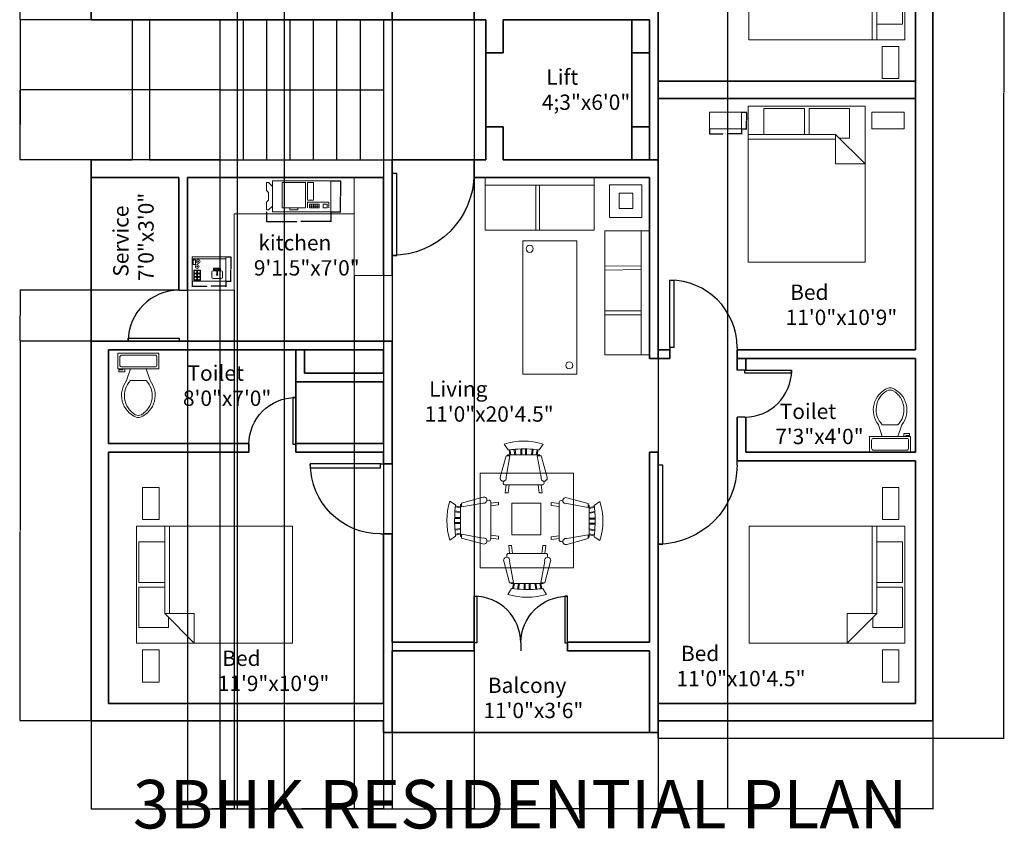
# Model space of a CAD drawing. Units: inches. Extents: x 108 to 613, y 1573 to 2319.
# Tile 1 of 11: x 108 to 613, y 1573 to 1989. Entities that reach past the tile are written whole.
import ezdxf

# ---------------------------------------------------------------- set-up
doc = ezdxf.new("R2010")
doc.units = ezdxf.units.IN
for name, color, linetype, lineweight in [('A-ANNO-DIMS', 2, 'Continuous', 18), ('A-AREA-IDEN', 3, 'Continuous', 18), ('A-EQPM', 2, 'Continuous', 18), ('A-FLOR-CASE', 6, 'Continuous', 18), ('A-FLOR-FIXT', 2, 'Continuous', 18), ('door', 4, 'Continuous', 25), ('furniture', 2, 'Continuous', 18), ('staircase', 7, 'Continuous', 25), ('text', 7, 'Continuous', 25), ('wall', 6, 'Continuous', 35)]:
    doc.layers.add(name, color=color, linetype=linetype, lineweight=lineweight)
doc.styles.get("Standard").update_dxf_attribs({"font": 'arial.ttf'})
doc.dimstyles.get("Standard").update_dxf_attribs({"dimtxt": 0.18, "dimasz": 0.18, "dimexe": 0.18, "dimexo": 0.0625, "dimgap": 0.09, "dimtad": 0, "dimtih": 1, "dimtoh": 1, "dimdec": 4, "dimzin": 0, "dimdsep": 46, "dimtxsty": 'Standard', "dimcen": 0.09, "dimadec": 0, "dimazin": 0, "dimtfac": 1, "dimtdec": 4, "dimtofl": 0, "dimtmove": 0, "dimatfit": 3, "dimfxl": 1, "dimtolj": 1, "dimtzin": 0, "dimarcsym": 0})

# ---------------------------------------------------------------- blocks, each defined once
blk = doc.blocks.new('*U2')
for p, q in [((0, 0), (0, -5)), ((30, 0), (30, -5))]:
    blk.add_line(p, q)
blk.add_lwpolyline([(0, 0), (0, 30), (1.75, 30), (1.75, 0)], close=True)
blk.add_arc((0, 0), 30, 0, 90)
blk = doc.blocks.new('Bed - Queen')
for p, q in [((0, -80.00003), (0, 0)), ((0, 0), (59.99999, 0)), ((59.99999, 0), (59.99999, -80.00003)), ((7.99999, -1.2), (28.79998, -1.2)), ((7.99999, -14.4), (7.99999, -1.2)), ((28.79998, -1.2), (28.79998, -14.4)), ((31.19999, -1.2), (51.99999, -1.2)), ((31.19999, -14.4), (31.19999, -1.2)), ((51.99999, -1.2), (51.99999, -16.4)), ((0, -14.4), (44.8, -14.4)), ((59.99999, -29.6), (44.8, -14.4)), ((44.8, -14.4), (44.8, -29.6)), ((44.8, -16.8), (0, -16.8)), ((51.99999, -16.4), (46.79936, -16.4)), ((44.8, -29.6), (59.99999, -29.6)), ((59.99999, -80.00003), (0, -80.00003))]:
    blk.add_line(p, q)
blk = doc.blocks.new('Copy Machine')
for p, q in [((0, 0), (0, -16)), ((30, 0), (0, 0)), ((30, -16), (30, 0)), ((-3, -1), (-3, -5)), ((-2, -1), (-3, -1)), ((-3, -5), (-2, -6)), ((0, -3), (-2, -1)), ((5, -1), (5, -14)), ((17, -1), (5, -1)), ((17, -14), (17, -1)), ((18, -1), (18, -10)), ((21, -1), (18, -1)), ((21, -10), (21, -1)), ((-3, -11), (-2, -10)), ((-2, -10), (-2, -6)), ((18, -10), (21, -10)), ((-3, -15), (-3, -11)), ((-2, -15), (-3, -15)), ((0, -13), (-2, -15)), ((5, -14), (17, -14)), ((9, -14), (9, -15)), ((9, -15), (13, -15)), ((13, -15), (13, -14)), ((18, -14), (18, -11)), ((18, -11), (29, -11)), ((24, -12), (19, -12)), ((19, -12), (19, -14)), ((24, -13), (19, -13)), ((19, -14), (24, -14)), ((20, -12), (20, -14)), ((21, -14), (21, -12)), ((22, -12), (22, -14)), ((23, -14), (23, -12)), ((24, -14), (24, -12)), ((28, -12), (26, -12)), ((26, -12), (26, -14)), ((26, -14), (28, -14)), ((28, -14), (28, -12)), ((29, -11), (29, -14)), ((0, -16), (30, -16))]:
    blk.add_line(p, q)
blk = doc.blocks.new('Wet Bar')
for p, q in [((0, 0), (36, 0)), ((0, -26), (0, 0)), ((36, 0), (36, -26)), ((0, -2), (36, -2)), ((3.5, -3), (1, -3)), ((1, -3), (1, -8)), ((1, -8), (3.5, -8)), ((3.5, -8), (3.5, -3)), ((2, -14.25), (9, -14.25)), ((2, -24.75), (2, -14.25)), ((2, -17.75), (9, -17.75)), ((5.5, -14.25), (5.5, -24.75)), ((9, -14.25), (9, -24.75)), ((26.2, -17.55), (26.2, -14.1284)), ((27.1001, -17.55), (27.1001, -14.1284)), ((36, -26), (0, -26)), ((9, -21.25), (2, -21.25)), ((9, -24.75), (2, -24.75))]:
    blk.add_line(p, q)
for points in [[(20.95, -21.75), (20.95, -16.05)], [(22.15, -14.85), (26.2, -14.85)], [(26.2, -14.25), (22.95, -14.25), (22.95, -12.2), (26.75, -12.2)], [(26.7487, -12.2), (30.3501, -12.2), (30.3501, -14.25), (27.1001, -14.25)], [(27.1001, -14.85), (31.15, -14.85)], [(32.3501, -16.05), (32.3501, -21.75)], [(31.15, -22.95), (22.15, -22.95)]]:
    blk.add_lwpolyline(points)
for centre, radius in [((5.5, -10.25), 2), ((6.5, -5), 2), ((5.5, -10.25), 0.5), ((6.5, -5), 0.5), ((3.75, -16), 1.5), ((3.75, -19.5), 1.5), ((7.25, -16), 1.5), ((7.25, -19.5), 1.5), ((24.25, -13.25), 0.5), ((26.65, -13.35), 0.9), ((26.65, -19.05), 0.6), ((29, -13.25), 0.5), ((3.75, -23), 1.5), ((7.25, -23), 1.5)]:
    blk.add_circle(centre, radius)
for centre, radius, start, end in [((22.2251, -16.125), 1.2772, 93.36646, 176.6335), ((26.65, -17.55), 0.45, 180, 0), ((31.075, -16.125), 1.2772, 3.366461, 86.63354), ((22.2251, -21.675), 1.2772, 183.3665, 266.6335), ((31.075, -21.675), 1.2772, 273.3665, 356.6335)]:
    blk.add_arc(centre, radius, start, end)
blk = doc.blocks.new('Toilet - top')
for p, q in [((9.5, -6), (9.5, -2)), ((-10, -8.5), (-8, -8.5)), ((-10, -9.5), (-10, -8.5)), ((-7, -9.5), (-10, -9.5)), ((-8, -8.5), (-8, -8)), ((-7, -8), (-7, -9.5)), ((-4, -8), (-6, -14)), ((4, -8), (6, -14)), ((4, -14), (-4, -14))]:
    blk.add_line(p, q)
blk.add_lwpolyline([(10.5, -8), (10.5, 0), (-10.5, 0), (-10.5, -8)], close=True)
for points in [[(-9.5, -2), (-9.5, -6)], [(8.5, -1), (-8.5, -1)], [(-8.5, -7), (8.5, -7)]]:
    blk.add_lwpolyline(points)
for centre, radius, start, end in [((-8.62, -1.88), 0.884, 81.8699, 188.1301), ((8.62, -1.88), 0.884, 351.8699, 98.1301), ((-8.62, -6.12), 0.884, 171.8699, 278.1301), ((8.62, -6.12), 0.884, 261.8699, 8.1301), ((3.52, -21.58), 12.17, 141.4691, 247.9714), ((4.2, -21.82), 11.33, 136.3677, 238.9468), ((-3.52, -21.58), 12.17, 292.0284, 38.5307), ((-4.2, -21.82), 11.33, 301.053, 43.6321), ((0, -27.88), 4, 245.7318, 294.2682), ((0, -29), 4, 254.8605, 285.1395)]:
    blk.add_arc(centre, radius, start, end)
blk = doc.blocks.new('Chair - Rocking')
for p, q in [((-8, -4.5), (-10, -1.5)), ((-7.5, -4.5), (-7, -7)), ((-6.5, -7), (-7.02225, -4.43)), ((-4.5, -7), (-4.96674, -4.19951)), ((-4, -7), (-4.40532, -4.16272)), ((-1.5, -4.05012), (-1.5, -7)), ((-1, -7), (-1, -4.05012)), ((1, -7), (1, -4.04655)), ((1.5, -4.05012), (1.5, -7)), ((4, -7), (4.40187, -4.18694)), ((4.5, -7), (4.96761, -4.19437)), ((6.5, -7), (7, -4.4057)), ((7.5, -4.5), (7, -7)), ((8, -4.5), (10, -1.5)), ((-9, -7.5), (-12, -18.49999)), ((-7, -7.5), (-9, -7.5)), ((-9, -18.49999), (-7, -7.5)), ((-8.23428, -6.99939), (-8.3093, -7.47958)), ((-8.23041, -7), (8.23915, -7)), ((7, -7.5), (9, -7.5)), ((9, -18.49999), (7, -7.5)), ((8.31071, -7.48854), (8.23449, -7.00073)), ((9, -7.5), (12, -18.49999)), ((-10.36644, -20.64523), (-10.5, -21.49999)), ((-9, -22.49999), (-9.5, -26.49999)), ((0, -22.49999), (-9.5, -22.49999)), ((-8, -26.49999), (-7.5, -22.49999)), ((0, -22.49999), (9.5, -22.49999)), ((8, -26.49999), (7.5, -22.49999)), ((9, -22.49999), (9.5, -26.49999)), ((10.5, -21.49999), (10.3575, -20.58798)), ((-9.5, -26.49999), (-8, -26.49999)), ((9.5, -26.49999), (8, -26.49999))]:
    blk.add_line(p, q)
for centre, radius, start, end in [((0, -34.08333), 34.08333, 72.93847, 107.0615), ((0, -68.25004), 64.25, 93.92211, 97.15267), ((0, -68.25004), 64.25, 82.84733, 93.92211), ((-10.5, -18.99999), 1.58114, 161.5651, 18.43495), ((10.5, -18.99999), 1.58114, 161.5651, 18.43495), ((-9.5, -21.49999), 1, 180, 270), ((9.5, -21.49999), 1, 270, 0)]:
    blk.add_arc(centre, radius, start, end)
blk = doc.blocks.new('NIGHTSTAND')
blk.add_lwpolyline([(0, 8.48), (16.5, 8.48), (16.5, 0), (0, 0)], close=True)
blk = doc.blocks.new('COFFEE-TABLE')
blk.add_lwpolyline([(0, 68.46), (27.63, 68.46), (27.63, 0), (0, 0)], close=True)
for centre, radius in [((23.79, 63.93), 1.79), ((3.47, 4.05), 1.83)]:
    blk.add_circle(centre, radius)
blk = doc.blocks.new('SOFA-3-SEAT')
for p, q in [((18.7, 63.66), (18.7, 0)), ((0.03, 43.08), (18.7, 43.08)), ((0.03, 41.08), (18.7, 41.08)), ((0, 18.17), (18.7, 17.89)), ((0.03, 20.17), (18.7, 19.89))]:
    blk.add_line(p, q)
blk.add_lwpolyline([(0.03, 63.66), (22.97, 63.66), (22.97, 0), (0.03, 0)], close=True)
blk = doc.blocks.new('SOFA-2-SEAT')
for p, q in [((25.99, 27.08), (25.99, 4.03)), ((27.99, 27.08), (27.99, 4.03)), ((55.98, 4.03), (0, 4.03))]:
    blk.add_line(p, q)
blk.add_lwpolyline([(0, 27.08), (55.98, 27.08), (55.98, 0), (0, 0)], close=True)
blk = doc.blocks.new('END-TABLE')
for points in [[(0, 16.91), (16.47, 16.91), (16.47, 0), (0, 0)], [(4.92, 12.21), (11.85, 12.21), (11.85, 4.34), (4.92, 4.34)]]:
    blk.add_lwpolyline(points, close=True)
blk = doc.blocks.new('DINING-TABLE')
for points in [[(0, 48.71), (48.06, 48.71), (48.06, 0), (0, 0)], [(16.26, 33.17), (31.3, 33.17), (31.3, 16.93), (16.26, 16.93)]]:
    blk.add_lwpolyline(points, close=True)
blk = doc.blocks.new('*D17')
at = {"layer": 'A-ANNO-DIMS', "color": 0, "lineweight": -2, "transparency": 16777216}
for p, q in [((462.07, 1932.51), (462.07, 1929.91)), ((478.57, 1932.51), (478.57, 1929.91)), ((462.25, 1930.09), (468.94, 1930.09)), ((478.39, 1930.09), (471.7, 1930.09))]:
    blk.add_line(p, q, dxfattribs=at)
at = {"layer": 'A-ANNO-DIMS', "color": 0, "transparency": 16777216}
for points in [[(462.25, 1930.12), (462.25, 1930.06), (462.07, 1930.09)], [(478.39, 1930.12), (478.39, 1930.06), (478.57, 1930.09)]]:
    blk.add_solid(points, dxfattribs=at)
at = {"layer": 'Defpoints', "color": 0, "transparency": 16777216}
for p in [(462.07, 1932.57), (478.57, 1932.57), (478.57, 1930.09)]:
    blk.add_point(p, dxfattribs=at)
at = {"layer": 'A-ANNO-DIMS', "color": 0, "transparency": 16777216, "insert": (470.32, 1930.09), "char_height": 0.18, "attachment_point": 5}
blk.add_mtext('\\A1;NIGHTSTAND 17 TYP.', dxfattribs=at)
blk = doc.blocks.new('*D18')
at = {"layer": 'A-ANNO-DIMS', "color": 0, "lineweight": -2, "transparency": 16777216}
for p, q in [((478.63, 1941.05), (481.23, 1941.05)), ((481.05, 1940.87), (481.05, 1936.99)), ((481.05, 1932.75), (481.05, 1936.63)), ((478.63, 1932.57), (481.23, 1932.57))]:
    blk.add_line(p, q, dxfattribs=at)
at = {"layer": 'A-ANNO-DIMS', "color": 0, "transparency": 16777216}
for points in [[(481.02, 1940.87), (481.08, 1940.87), (481.05, 1941.05)], [(481.02, 1932.75), (481.08, 1932.75), (481.05, 1932.57)]]:
    blk.add_solid(points, dxfattribs=at)
at = {"layer": 'Defpoints', "color": 0, "transparency": 16777216}
for p in [(478.57, 1941.05), (481.05, 1941.05), (478.57, 1932.57)]:
    blk.add_point(p, dxfattribs=at)
at = {"layer": 'A-ANNO-DIMS', "color": 0, "transparency": 16777216, "insert": (481.05, 1936.81), "char_height": 0.18, "attachment_point": 5}
blk.add_mtext('\\A1;8 TYP.', dxfattribs=at)
blk = doc.blocks.new('*D25')
at = {"layer": 'A-ANNO-DIMS', "color": 0, "lineweight": -2, "transparency": 16777216}
for p, q in [((234.84, 1889.9), (234.84, 1884.83)), ((267.84, 1889.9), (267.84, 1884.83)), ((235.02, 1885.01), (250.3, 1885.01)), ((267.66, 1885.01), (252.38, 1885.01))]:
    blk.add_line(p, q, dxfattribs=at)
at = {"layer": 'A-ANNO-DIMS', "color": 0, "transparency": 16777216}
for points in [[(235.02, 1885.04), (235.02, 1884.98), (234.84, 1885.01)], [(267.66, 1885.04), (267.66, 1884.98), (267.84, 1885.01)]]:
    blk.add_solid(points, dxfattribs=at)
at = {"layer": 'Defpoints', "color": 0, "transparency": 16777216}
for p in [(234.84, 1889.96), (267.84, 1889.96), (267.84, 1885.01)]:
    blk.add_point(p, dxfattribs=at)
at = {"layer": 'A-ANNO-DIMS', "color": 0, "transparency": 16777216, "insert": (251.34, 1885.01), "char_height": 0.18, "attachment_point": 5}
blk.add_mtext('\\A1;COPIER 33 TYP.', dxfattribs=at)
blk = doc.blocks.new('*D26')
at = {"layer": 'A-ANNO-DIMS', "color": 0, "lineweight": -2, "transparency": 16777216}
for p, q in [((267.9, 1905.96), (272.97, 1905.96)), ((272.79, 1905.78), (272.79, 1898.14)), ((272.79, 1890.14), (272.79, 1897.78)), ((267.9, 1889.96), (272.97, 1889.96))]:
    blk.add_line(p, q, dxfattribs=at)
at = {"layer": 'A-ANNO-DIMS', "color": 0, "transparency": 16777216}
for points in [[(272.76, 1905.78), (272.82, 1905.78), (272.79, 1905.96)], [(272.76, 1890.14), (272.82, 1890.14), (272.79, 1889.96)]]:
    blk.add_solid(points, dxfattribs=at)
at = {"layer": 'Defpoints', "color": 0, "transparency": 16777216}
for p in [(267.84, 1905.96), (272.79, 1905.96), (267.84, 1889.96)]:
    blk.add_point(p, dxfattribs=at)
at = {"layer": 'A-ANNO-DIMS', "color": 0, "transparency": 16777216, "insert": (272.79, 1897.96), "char_height": 0.18, "attachment_point": 5}
blk.add_mtext('\\A1;16 TYP.', dxfattribs=at)
blk = doc.blocks.new('*D27')
at = {"layer": 'A-ANNO-DIMS', "color": 0, "lineweight": -2, "transparency": 16777216}
for p, q in [((196.59, 1854.26), (196.59, 1851.54)), ((196.77, 1851.72), (204.13, 1851.72)), ((213.76, 1851.72), (206.4, 1851.72)), ((213.94, 1854.26), (213.94, 1851.54))]:
    blk.add_line(p, q, dxfattribs=at)
at = {"layer": 'A-ANNO-DIMS', "color": 0, "transparency": 16777216}
for points in [[(196.77, 1851.75), (196.77, 1851.69), (196.59, 1851.72)], [(213.76, 1851.75), (213.76, 1851.69), (213.94, 1851.72)]]:
    blk.add_solid(points, dxfattribs=at)
at = {"layer": 'Defpoints', "color": 0, "transparency": 16777216}
for p in [(196.59, 1854.32), (213.94, 1854.32), (213.94, 1851.72)]:
    blk.add_point(p, dxfattribs=at)
at = {"layer": 'A-ANNO-DIMS', "color": 0, "transparency": 16777216, "insert": (205.27, 1851.72), "char_height": 0.18, "attachment_point": 5}
blk.add_mtext('\\A1;WET BAR 17 TYP.', dxfattribs=at)
blk = doc.blocks.new('*D28')
at = {"layer": 'A-ANNO-DIMS', "color": 0, "lineweight": -2, "transparency": 16777216}
for p, q in [((214, 1866.85), (216.72, 1866.85)), ((216.54, 1866.67), (216.54, 1860.77)), ((216.54, 1854.5), (216.54, 1860.4)), ((214, 1854.32), (216.72, 1854.32))]:
    blk.add_line(p, q, dxfattribs=at)
at = {"layer": 'A-ANNO-DIMS', "color": 0, "transparency": 16777216}
for points in [[(216.51, 1866.67), (216.57, 1866.67), (216.54, 1866.85)], [(216.51, 1854.5), (216.57, 1854.5), (216.54, 1854.32)]]:
    blk.add_solid(points, dxfattribs=at)
at = {"layer": 'Defpoints', "color": 0, "transparency": 16777216}
for p in [(213.94, 1866.85), (216.54, 1866.85), (213.94, 1854.32)]:
    blk.add_point(p, dxfattribs=at)
at = {"layer": 'A-ANNO-DIMS', "color": 0, "transparency": 16777216, "insert": (216.54, 1860.59), "char_height": 0.18, "attachment_point": 5}
blk.add_mtext('\\A1;13 TYP.', dxfattribs=at)
blk = doc.blocks.new('*D39')
at = {"layer": 'A-ANNO-DIMS', "color": 0, "lineweight": -2, "transparency": 16777216}
for p, q in [((144.78, 1628.55), (144.78, 1583.23)), ((576.78, 1628.55), (576.78, 1583.23)), ((144.96, 1583.41), (360.48, 1583.41)), ((576.6, 1583.41), (361.07, 1583.41))]:
    blk.add_line(p, q, dxfattribs=at)
at = {"layer": 'A-ANNO-DIMS', "color": 0, "transparency": 16777216}
for points in [[(144.96, 1583.44), (144.96, 1583.38), (144.78, 1583.41)], [(576.6, 1583.44), (576.6, 1583.38), (576.78, 1583.41)]]:
    blk.add_solid(points, dxfattribs=at)
at = {"layer": 'Defpoints', "color": 0, "transparency": 16777216}
for p in [(144.78, 1628.61), (576.78, 1628.61), (576.78, 1583.41)]:
    blk.add_point(p, dxfattribs=at)
at = {"layer": 'A-ANNO-DIMS', "color": 0, "transparency": 16777216, "insert": (360.78, 1583.41), "char_height": 0.18, "attachment_point": 5}
blk.add_mtext('\\A1;432', dxfattribs=at)
blk = doc.blocks.new('*D40')
at = {"layer": 'A-ANNO-DIMS', "color": 0, "lineweight": -2, "transparency": 16777216}
for p, q in [((435.84, 2282.61), (613.31, 2282.61)), ((613.13, 2282.43), (613.13, 1951.37)), ((613.13, 1619.94), (613.13, 1951.01)), ((435.84, 1619.76), (613.31, 1619.76))]:
    blk.add_line(p, q, dxfattribs=at)
at = {"layer": 'A-ANNO-DIMS', "color": 0, "transparency": 16777216}
for points in [[(613.1, 2282.43), (613.16, 2282.43), (613.13, 2282.61)], [(613.1, 1619.94), (613.16, 1619.94), (613.13, 1619.76)]]:
    blk.add_solid(points, dxfattribs=at)
at = {"layer": 'Defpoints', "color": 0, "transparency": 16777216}
for p in [(435.78, 2282.61), (613.13, 2282.61), (435.78, 1619.76)]:
    blk.add_point(p, dxfattribs=at)
at = {"layer": 'A-ANNO-DIMS', "color": 0, "transparency": 16777216, "insert": (613.13, 1951.19), "char_height": 0.18, "attachment_point": 5}
blk.add_mtext('\\A1;662.8', dxfattribs=at)
blk = doc.blocks.new('*D43')
at = {"layer": 'A-ANNO-DIMS', "color": 0, "lineweight": -2, "transparency": 16777216}
for p, q in [((144.71, 1823.61), (108.25, 1823.61)), ((108.43, 1823.43), (108.43, 1726.29)), ((108.43, 1628.79), (108.43, 1725.93)), ((144.71, 1628.61), (108.25, 1628.61))]:
    blk.add_line(p, q, dxfattribs=at)
at = {"layer": 'A-ANNO-DIMS', "color": 0, "transparency": 16777216}
for points in [[(108.4, 1823.43), (108.46, 1823.43), (108.43, 1823.61)], [(108.4, 1628.79), (108.46, 1628.79), (108.43, 1628.61)]]:
    blk.add_solid(points, dxfattribs=at)
at = {"layer": 'Defpoints', "color": 0, "transparency": 16777216}
for p in [(108.43, 1823.61), (144.78, 1823.61), (144.78, 1628.61)]:
    blk.add_point(p, dxfattribs=at)
at = {"layer": 'A-ANNO-DIMS', "color": 0, "transparency": 16777216, "insert": (108.43, 1726.11), "char_height": 0.18, "attachment_point": 5}
blk.add_mtext('\\A1;195', dxfattribs=at)
blk = doc.blocks.new('*D44')
at = {"layer": 'A-ANNO-DIMS', "color": 0, "lineweight": -2, "transparency": 16777216}
for p, q in [((144.71, 1988.61), (108.25, 1988.61)), ((108.43, 1988.43), (108.43, 1952.79)), ((108.43, 1916.79), (108.43, 1952.43)), ((144.71, 1916.61), (108.25, 1916.61))]:
    blk.add_line(p, q, dxfattribs=at)
at = {"layer": 'A-ANNO-DIMS', "color": 0, "transparency": 16777216}
for points in [[(108.4, 1988.43), (108.46, 1988.43), (108.43, 1988.61)], [(108.4, 1916.79), (108.46, 1916.79), (108.43, 1916.61)]]:
    blk.add_solid(points, dxfattribs=at)
at = {"layer": 'Defpoints', "color": 0, "transparency": 16777216}
for p in [(108.43, 1988.61), (144.78, 1988.61), (144.78, 1916.61)]:
    blk.add_point(p, dxfattribs=at)
at = {"layer": 'A-ANNO-DIMS', "color": 0, "transparency": 16777216, "insert": (108.43, 1952.61), "char_height": 0.18, "attachment_point": 5}
blk.add_mtext('\\A1;72', dxfattribs=at)
blk = doc.blocks.new('*D45')
at = {"layer": 'A-ANNO-DIMS', "color": 0, "lineweight": -2, "transparency": 16777216}
for p, q in [((144.71, 2276.61), (108.25, 2276.61)), ((108.43, 2276.43), (108.43, 2132.79)), ((108.43, 1988.79), (108.43, 2132.43)), ((144.71, 1988.61), (108.25, 1988.61))]:
    blk.add_line(p, q, dxfattribs=at)
at = {"layer": 'A-ANNO-DIMS', "color": 0, "transparency": 16777216}
for points in [[(108.4, 2276.43), (108.46, 2276.43), (108.43, 2276.61)], [(108.4, 1988.79), (108.46, 1988.79), (108.43, 1988.61)]]:
    blk.add_solid(points, dxfattribs=at)
at = {"layer": 'Defpoints', "color": 0, "transparency": 16777216}
for p in [(108.43, 2276.61), (144.78, 2276.61), (144.78, 1988.61)]:
    blk.add_point(p, dxfattribs=at)
at = {"layer": 'A-ANNO-DIMS', "color": 0, "transparency": 16777216, "insert": (108.43, 2132.61), "char_height": 0.18, "attachment_point": 5}
blk.add_mtext('\\A1;288', dxfattribs=at)
blk = doc.blocks.new('*D48')
at = {"layer": 'A-ANNO-DIMS', "color": 0, "lineweight": -2, "transparency": 16777216}
for p, q in [((299.28, 1988.55), (299.28, 1583.23)), ((341.28, 1988.55), (341.28, 1583.23)), ((299.46, 1583.41), (320.05, 1583.41)), ((341.1, 1583.41), (320.5, 1583.41))]:
    blk.add_line(p, q, dxfattribs=at)
at = {"layer": 'A-ANNO-DIMS', "color": 0, "transparency": 16777216}
for points in [[(299.46, 1583.44), (299.46, 1583.38), (299.28, 1583.41)], [(341.1, 1583.44), (341.1, 1583.38), (341.28, 1583.41)]]:
    blk.add_solid(points, dxfattribs=at)
at = {"layer": 'Defpoints', "color": 0, "transparency": 16777216}
for p in [(299.28, 1988.61), (341.28, 1988.61), (341.28, 1583.41)]:
    blk.add_point(p, dxfattribs=at)
at = {"layer": 'A-ANNO-DIMS', "color": 0, "transparency": 16777216, "insert": (320.28, 1583.41), "char_height": 0.18, "attachment_point": 5}
blk.add_mtext('\\A1;42', dxfattribs=at)
blk = doc.blocks.new('*D49')
at = {"layer": 'A-ANNO-DIMS', "color": 0, "lineweight": -2, "transparency": 16777216}
for p, q in [((219.78, 2126.55), (219.78, 1583.23)), ((243.78, 2126.55), (243.78, 1583.23)), ((219.96, 1583.41), (231.56, 1583.41)), ((243.6, 1583.41), (232, 1583.41))]:
    blk.add_line(p, q, dxfattribs=at)
at = {"layer": 'A-ANNO-DIMS', "color": 0, "transparency": 16777216}
for points in [[(219.96, 1583.44), (219.96, 1583.38), (219.78, 1583.41)], [(243.6, 1583.44), (243.6, 1583.38), (243.78, 1583.41)]]:
    blk.add_solid(points, dxfattribs=at)
at = {"layer": 'Defpoints', "color": 0, "transparency": 16777216}
for p in [(219.78, 2126.61), (243.78, 2126.61), (243.78, 1583.41)]:
    blk.add_point(p, dxfattribs=at)
at = {"layer": 'A-ANNO-DIMS', "color": 0, "transparency": 16777216, "insert": (231.78, 1583.41), "char_height": 0.18, "attachment_point": 5}
blk.add_mtext('\\A1;24', dxfattribs=at)
blk = doc.blocks.new('*D50')
at = {"layer": 'A-ANNO-DIMS', "color": 0, "lineweight": -2, "transparency": 16777216}
for p, q in [((435.78, 2137.91), (435.78, 1583.23)), ((471.43, 2138.55), (471.43, 1583.23)), ((435.96, 1583.41), (453.21, 1583.41)), ((471.25, 1583.41), (454, 1583.41))]:
    blk.add_line(p, q, dxfattribs=at)
at = {"layer": 'A-ANNO-DIMS', "color": 0, "transparency": 16777216}
for points in [[(435.96, 1583.44), (435.96, 1583.38), (435.78, 1583.41)], [(471.25, 1583.44), (471.25, 1583.38), (471.43, 1583.41)]]:
    blk.add_solid(points, dxfattribs=at)
at = {"layer": 'Defpoints', "color": 0, "transparency": 16777216}
for p in [(435.78, 2137.98), (471.43, 2138.61), (471.43, 1583.41)]:
    blk.add_point(p, dxfattribs=at)
at = {"layer": 'A-ANNO-DIMS', "color": 0, "transparency": 16777216, "insert": (453.6, 1583.41), "char_height": 0.18, "attachment_point": 5}
blk.add_mtext('\\A1;35.66', dxfattribs=at)
blk = doc.blocks.new('*D51')
at = {"layer": 'A-ANNO-DIMS', "color": 0, "lineweight": -2, "transparency": 16777216}
for p, q in [((194.28, 1849.67), (194.28, 1583.23)), ((218.24, 1849.67), (218.24, 1583.23)), ((194.46, 1583.41), (205.79, 1583.41)), ((218.06, 1583.41), (206.72, 1583.41))]:
    blk.add_line(p, q, dxfattribs=at)
at = {"layer": 'A-ANNO-DIMS', "color": 0, "transparency": 16777216}
for points in [[(194.46, 1583.44), (194.46, 1583.38), (194.28, 1583.41)], [(218.06, 1583.44), (218.06, 1583.38), (218.24, 1583.41)]]:
    blk.add_solid(points, dxfattribs=at)
at = {"layer": 'Defpoints', "color": 0, "transparency": 16777216}
for p in [(194.28, 1849.73), (218.24, 1849.73), (218.24, 1583.41)]:
    blk.add_point(p, dxfattribs=at)
at = {"layer": 'A-ANNO-DIMS', "color": 0, "transparency": 16777216, "insert": (206.26, 1583.41), "char_height": 0.18, "attachment_point": 5}
blk.add_mtext('\\A1;23.963', dxfattribs=at)
blk = doc.blocks.new('*D52')
at = {"layer": 'A-ANNO-DIMS', "color": 0, "lineweight": -2, "transparency": 16777216}
for p, q in [((279.84, 1857.2), (279.84, 1583.23)), ((294.78, 1857.2), (294.78, 1583.23)), ((280.02, 1583.41), (286.92, 1583.41)), ((294.6, 1583.41), (287.69, 1583.41))]:
    blk.add_line(p, q, dxfattribs=at)
at = {"layer": 'A-ANNO-DIMS', "color": 0, "transparency": 16777216}
for points in [[(280.02, 1583.44), (280.02, 1583.38), (279.84, 1583.41)], [(294.6, 1583.44), (294.6, 1583.38), (294.78, 1583.41)]]:
    blk.add_solid(points, dxfattribs=at)
at = {"layer": 'Defpoints', "color": 0, "transparency": 16777216}
for p in [(279.84, 1857.27), (294.78, 1857.27), (294.78, 1583.41)]:
    blk.add_point(p, dxfattribs=at)
at = {"layer": 'A-ANNO-DIMS', "color": 0, "transparency": 16777216, "insert": (287.31, 1583.41), "char_height": 0.18, "attachment_point": 5}
blk.add_mtext('\\A1;14.94', dxfattribs=at)
blk = doc.blocks.new('*D53')
at = {"layer": 'A-ANNO-DIMS', "color": 0, "lineweight": -2, "transparency": 16777216}
for p, q in [((189.71, 1849.73), (108.25, 1849.73)), ((108.43, 1849.55), (108.43, 1836.85)), ((108.43, 1823.79), (108.43, 1836.49)), ((189.86, 1823.61), (108.25, 1823.61))]:
    blk.add_line(p, q, dxfattribs=at)
at = {"layer": 'A-ANNO-DIMS', "color": 0, "transparency": 16777216}
for points in [[(108.4, 1849.55), (108.46, 1849.55), (108.43, 1849.73)], [(108.4, 1823.79), (108.46, 1823.79), (108.43, 1823.61)]]:
    blk.add_solid(points, dxfattribs=at)
at = {"layer": 'Defpoints', "color": 0, "transparency": 16777216}
for p in [(108.43, 1849.73), (189.78, 1849.73), (189.92, 1823.61)]:
    blk.add_point(p, dxfattribs=at)
at = {"layer": 'A-ANNO-DIMS', "color": 0, "transparency": 16777216, "insert": (108.43, 1836.67), "char_height": 0.18, "attachment_point": 5}
blk.add_mtext('\\A1;26.12', dxfattribs=at)
blk = doc.blocks.new('*D54')
at = {"layer": 'A-ANNO-DIMS', "color": 0, "lineweight": -2, "transparency": 16777216}
for p, q in [((210.78, 1988.55), (210.78, 1583.23)), ((294.78, 1988.55), (294.78, 1583.23)), ((210.96, 1583.41), (252.56, 1583.41)), ((294.6, 1583.41), (252.99, 1583.41))]:
    blk.add_line(p, q, dxfattribs=at)
at = {"layer": 'A-ANNO-DIMS', "color": 0, "transparency": 16777216}
for points in [[(210.96, 1583.44), (210.96, 1583.38), (210.78, 1583.41)], [(294.6, 1583.44), (294.6, 1583.38), (294.78, 1583.41)]]:
    blk.add_solid(points, dxfattribs=at)
at = {"layer": 'Defpoints', "color": 0, "transparency": 16777216}
for p in [(210.78, 1988.61), (294.78, 1988.61), (294.78, 1583.41)]:
    blk.add_point(p, dxfattribs=at)
at = {"layer": 'A-ANNO-DIMS', "color": 0, "transparency": 16777216, "insert": (252.78, 1583.41), "char_height": 0.18, "attachment_point": 5}
blk.add_mtext('\\A1;84', dxfattribs=at)
blk = doc.blocks.new('*D55')
at = {"layer": 'A-ANNO-DIMS', "color": 0, "lineweight": -2, "transparency": 16777216}
for p, q in [((210.71, 1952.61), (108.25, 1952.61)), ((108.43, 1952.43), (108.43, 1934.79)), ((108.43, 1916.79), (108.43, 1934.43)), ((210.71, 1916.61), (108.25, 1916.61))]:
    blk.add_line(p, q, dxfattribs=at)
at = {"layer": 'A-ANNO-DIMS', "color": 0, "transparency": 16777216}
for points in [[(108.4, 1952.43), (108.46, 1952.43), (108.43, 1952.61)], [(108.4, 1916.79), (108.46, 1916.79), (108.43, 1916.61)]]:
    blk.add_solid(points, dxfattribs=at)
at = {"layer": 'Defpoints', "color": 0, "transparency": 16777216}
for p in [(210.78, 1952.61), (108.43, 1916.61), (210.78, 1916.61)]:
    blk.add_point(p, dxfattribs=at)
at = {"layer": 'A-ANNO-DIMS', "color": 0, "transparency": 16777216, "insert": (108.43, 1934.61), "char_height": 0.18, "attachment_point": 5}
blk.add_mtext('\\A1;36', dxfattribs=at)

msp = doc.modelspace()

# ---------------------------------------------------------------- linework, layer by layer
at = {"layer": 'A-FLOR-CASE'}
for p, q in [((279.8364, 1907.6125), (279.8364, 1857.2657)), ((218.2385, 1888.9466), (279.8364, 1888.9466)), ((218.2385, 1888.9466), (218.2385, 1849.7306)), ((279.8364, 1857.2657), (299.2753, 1857.2657)), ((189.7753, 1849.7306), (218.2385, 1849.7306))]:
    msp.add_line(p, q, dxfattribs=at)
at = {"layer": 'staircase'}
for p, q in [((165.7753, 1988.6125), (165.7753, 1916.6125)), ((174.7753, 1988.6125), (174.7753, 1916.6125)), ((174.7753, 1988.6125), (299.2753, 1988.6125)), ((210.7753, 1988.6125), (210.7753, 1916.6125)), ((222.7753, 1988.6125), (222.7753, 1916.6125)), ((234.7753, 1988.6125), (234.7753, 1916.6125)), ((246.7753, 1988.6125), (246.7753, 1916.6125)), ((258.7753, 1988.6125), (258.7753, 1916.6125)), ((270.7753, 1988.6125), (270.7753, 1916.6125)), ((282.7753, 1988.6125), (282.7753, 1916.6125)), ((294.7753, 1988.6125), (294.7753, 1916.6125)), ((210.7753, 1952.6125), (294.7753, 1952.6125)), ((174.7753, 1916.6125), (299.2753, 1916.6125))]:
    msp.add_line(p, q, dxfattribs=at)
at = {"layer": 'wall'}
for p, q in [((144.7753, 2276.6125), (144.7753, 1988.6125)), ((576.7753, 2276.6125), (576.7753, 1628.6125)), ((299.2753, 2096.6125), (299.2753, 1988.6125)), ((435.7753, 2092.1125), (435.7753, 1814.6125)), ((567.7753, 2081.6125), (567.7753, 1819.1125)), ((341.2753, 1988.6125), (341.2753, 1997.6125)), ((144.7753, 1988.6125), (165.7753, 1988.6125)), ((153.7753, 1988.6125), (299.2753, 1988.6125)), ((294.7753, 1988.6125), (347.2753, 1988.6125)), ((341.2753, 1988.6125), (347.2753, 1988.6125)), ((347.2753, 1988.6125), (347.2753, 1971.6125)), ((347.2753, 1988.6125), (347.2753, 1916.6125)), ((356.2753, 1988.6125), (356.2753, 1971.6125)), ((356.2753, 1988.6125), (431.2753, 1988.6125)), ((422.2753, 1988.6125), (422.2753, 1916.6125)), ((431.2753, 1988.6125), (431.2753, 1916.6125)), ((347.2753, 1971.6125), (356.2753, 1971.6125)), ((422.2753, 1971.6125), (431.2753, 1971.6125)), ((435.7753, 1957.1125), (567.7753, 1957.1125)), ((435.7753, 1948.1125), (567.7753, 1948.1125)), ((435.7753, 1948.1125), (435.7753, 1819.1125)), ((347.2753, 1933.6125), (356.2753, 1933.6125)), ((347.2753, 1933.6125), (347.2753, 1916.6125)), ((356.2753, 1933.6125), (356.2753, 1916.6125)), ((422.2753, 1933.6125), (431.2753, 1933.6125)), ((144.7753, 1916.6125), (165.7753, 1916.6125)), ((144.7753, 1916.6125), (144.7753, 1628.6125)), ((299.2753, 1916.6125), (299.2753, 1857.2657)), ((347.2753, 1916.6125), (299.2753, 1916.6125)), ((341.2753, 1916.6125), (347.2753, 1916.6125)), ((341.2753, 1907.6125), (341.2753, 1916.6125)), ((356.2753, 1916.6125), (431.2753, 1916.6125)), ((431.2753, 1916.6125), (435.7753, 1916.6125)), ((144.7753, 1907.6125), (189.7753, 1907.6125)), ((189.7753, 1849.7306), (189.7753, 1907.6125)), ((194.2753, 1849.7306), (194.2753, 1907.6125)), ((194.2753, 1907.6125), (294.7753, 1907.6125)), ((294.7753, 1907.6125), (294.7753, 1857.2657)), ((341.2753, 1907.6125), (431.2753, 1907.6125)), ((431.2753, 1907.6125), (431.2753, 1814.6125)), ((144.7753, 1823.6125), (299.2753, 1823.6125)), ((299.2753, 1823.6125), (299.2753, 1760.6125)), ((153.7753, 1819.1125), (294.7753, 1819.1125)), ((153.7753, 1819.1125), (153.7753, 1771.1125)), ((249.7753, 1819.1125), (249.7753, 1766.6125)), ((254.2753, 1819.1125), (254.2753, 1807.1125)), ((294.7753, 1819.1125), (294.7753, 1807.1125)), ((431.2753, 1814.6125), (441.7753, 1814.6125)), ((435.7753, 1819.1125), (441.7753, 1819.1125)), ((441.7753, 1819.1125), (441.7753, 1814.6125)), ((476.2753, 1819.1125), (476.2753, 1814.6125)), ((476.2753, 1819.1125), (567.7753, 1819.1125)), ((476.2753, 1814.6125), (476.2753, 1808.6125)), ((476.2753, 1814.6125), (567.7753, 1814.6125)), ((480.7753, 1814.6125), (480.7753, 1808.6125)), ((567.7753, 1814.6125), (567.7753, 1766.6125)), ((254.2753, 1807.1125), (294.7753, 1807.1125)), ((249.7753, 1802.6125), (294.7753, 1802.6125)), ((294.7753, 1802.6125), (294.7753, 1771.1125)), ((476.2753, 1784.6125), (476.2753, 1762.1125)), ((480.7753, 1784.6177), (480.7753, 1766.6125)), ((153.7753, 1771.1125), (225.7842, 1771.1125)), ((225.7842, 1771.1125), (225.7842, 1766.6125)), ((249.7753, 1771.1125), (294.7753, 1771.1125)), ((153.7753, 1766.6125), (225.7842, 1766.6125)), ((153.7753, 1766.6125), (153.7753, 1637.6125)), ((249.7753, 1766.6125), (294.7753, 1766.6125)), ((294.7753, 1766.6125), (294.7753, 1760.6125)), ((431.2753, 1766.6125), (435.7753, 1766.6125)), ((431.2753, 1766.6125), (431.2753, 1669.1125)), ((435.7753, 1766.6125), (435.7753, 1637.6125)), ((435.7753, 1766.6125), (435.7753, 1619.7647)), ((480.7753, 1766.6125), (567.7753, 1766.6125)), ((294.7753, 1760.6125), (299.2753, 1760.6125)), ((476.2753, 1762.1125), (567.7753, 1762.1125)), ((567.7753, 1762.1125), (567.7753, 1637.6125)), ((294.7753, 1724.6125), (299.2753, 1724.6125)), ((294.7753, 1724.6125), (294.7753, 1637.6125)), ((299.2753, 1724.6125), (299.2753, 1669.1125)), ((299.2753, 1669.1125), (341.2753, 1669.1125)), ((341.2753, 1664.6125), (341.2753, 1669.1125)), ((389.2753, 1664.6125), (389.2753, 1669.1125)), ((389.2753, 1669.1125), (431.2753, 1669.1125)), ((299.2753, 1664.6125), (341.2753, 1664.6125)), ((299.2753, 1664.6125), (299.2753, 1622.6125)), ((389.2753, 1664.6125), (431.2753, 1664.6125)), ((431.2753, 1664.6125), (431.2753, 1622.6125)), ((153.7753, 1637.6125), (294.7753, 1637.6125)), ((435.7753, 1637.6125), (567.7753, 1637.6125)), ((144.7753, 1628.6125), (294.7753, 1628.6125)), ((294.7753, 1628.6125), (294.7753, 1622.6125)), ((435.7753, 1628.6125), (576.7753, 1628.6125)), ((435.7753, 1628.6125), (435.7753, 1622.6125)), ((294.7753, 1622.6125), (435.7753, 1622.6125))]:
    msp.add_line(p, q, dxfattribs=at)

# ---------------------------------------------------------------- block references
at = {"layer": 'A-EQPM'}
msp.add_blockref('Copy Machine', (237.84, 1905.9581), dxfattribs=at)
at = {"layer": 'A-FLOR-FIXT', "xscale": 0.4817065936809276, "yscale": 0.4817065936809276, "zscale": 0.4817065936809276}
msp.add_blockref('Wet Bar', (196.5946, 1866.8483), dxfattribs=at)
at = {"layer": 'A-FLOR-FIXT'}
msp.add_blockref('Toilet - top', (169.0158, 1817.3563), dxfattribs=at)
at = {"layer": 'A-FLOR-FIXT', "rotation": 180}
msp.add_blockref('Toilet - top', (554.823, 1766.6125), dxfattribs=at)
at = {"layer": 'door'}
for p, xscale, yscale, zscale, rotation in [((299.2753, 1909.6125), -1.4, 1.4, 1.4, 180), ((189.9223, 1823.6125), 0.870603593816971, 0.870603593816971, 0.870603593816971, 89.99999999999991), ((480.2753, 1808.6125), 0.8, 0.8, 0.8, 270), ((435.7753, 1759.8625), -1.350000000000012, 1.350000000000012, 1.350000000000012, 180), ((293.2753, 1760.6125), -1.200000000000007, 1.200000000000007, 1.200000000000007, 90)]:
    msp.add_blockref('*U2', p, dxfattribs=dict(at, xscale=xscale, yscale=yscale, zscale=zscale, rotation=rotation))
for p, xscale, yscale, zscale in [((441.7753, 1820.3625), 1.149999999999999, 1.149999999999999, 1.149999999999999), ((249.7753, 1770.6125), -0.8, 0.8, 0.8), ((341.2753, 1668.6125), 0.8, 0.8, 0.8), ((389.2753, 1668.6125), -0.8, 0.8, 0.8)]:
    msp.add_blockref('*U2', p, dxfattribs=dict(at, xscale=xscale, yscale=yscale, zscale=zscale))
at = {"layer": 'furniture', "xscale": -1}
for p, rotation in [((562.378, 1978.3393), 270), ((168.1312, 1728.5051), 90)]:
    msp.add_blockref('Bed - Queen', p, dxfattribs=dict(at, rotation=rotation))
at = {"layer": 'furniture', "extrusion": (0, 0, -1), "zscale": -1}
for name, p, rotation in [('NIGHTSTAND', (-550.8088, 1958.3693), 89.9999999999982), ('SOFA-2-SEAT', (-346.962, 1907.613), 180), ('END-TABLE', (-410.889, 1903.892), 180), ('SOFA-3-SEAT', (-408.31, 1880.192), 180), ('COFFEE-TABLE', (-366.385, 1875.049), 180), ('NIGHTSTAND', (-179.7004, 1748.475), 269.9999999999979), ('NIGHTSTAND', (-179.7004, 1665.0689), 269.9999999999985)]:
    msp.add_blockref(name, p, dxfattribs=dict(at, rotation=rotation))
at = {"layer": 'furniture'}
for name, p in [('NIGHTSTAND', (462.0695, 1932.5691)), ('Bed - Queen', (482.0394, 1944.1384)), ('NIGHTSTAND', (545.4756, 1932.5691)), ('Chair - Rocking', (366.7413, 1772.2457)), ('DINING-TABLE', (344.357, 1707.143))]:
    msp.add_blockref(name, p, dxfattribs=at)
for name, p, rotation in [('NIGHTSTAND', (550.8503, 1748.475), 269.9999999999977), ('Chair - Rocking', (327.3278, 1731.4618), 90), ('Chair - Rocking', (407.4365, 1731.1892), 270), ('Bed - Queen', (562.4195, 1728.5051), 270), ('Chair - Rocking', (368.5653, 1692.0767), 180), ('NIGHTSTAND', (550.8503, 1665.0689), 269.9999999999982)]:
    msp.add_blockref(name, p, dxfattribs=dict(at, rotation=rotation))

# ---------------------------------------------------------------- texts
at = {"layer": 'A-AREA-IDEN'}
for s, height, p in [('Lift', 7.87346, (378.4208, 1955.2107)), ('4;3"x6\'0"', 7.87346, (376.1125, 1942.3048)), ('kitchen', 7.87346, (230.6046, 1870.1685)), ('9\'1.5"x7\'0"', 7.873465, (228.2963, 1857.2627)), ('Bed', 7.87346, (503.518, 1844.7721)), ('11\'0"x10\'9"', 7.873465, (501.2096, 1831.8662)), ('Toilet', 7.87346, (194.2137, 1803.2397)), ('Living', 7.87346, (318.2247, 1795.1273)), ('8\'0"x7\'0"', 7.87346, (191.9054, 1790.3339)), ('11\'0"x20\'4.5"', 7.873465, (315.9164, 1782.2214)), ('Toilet', 7.87346, (498.1832, 1783.622)), ('7\'3"x4\'0"', 7.87346, (495.8748, 1770.7161)), ('Bed', 7.87346, (447.4925, 1659.3203)), ('Bed', 7.87346, (212.0755, 1656.8347)), ('11\'0"x10\'4.5"', 7.873465, (445.1842, 1646.4145)), ('11\'9"x10\'9"', 7.873465, (209.7672, 1643.9288)), ('Balcony', 7.87346, (348.3807, 1642.9425)), ('11\'0"x3\'6"', 7.87346, (346.0723, 1630.0367))]:
    msp.add_text(s, height=height, dxfattribs=at).set_placement(p)
for s, p in [('7\'0"x3\'0"', (176.87, 1854.3761)), ('Service', (163.9641, 1856.6845))]:
    msp.add_text(s, height=7.87346, rotation=90, dxfattribs=at).set_placement(p)
at = {"layer": 'text'}
msp.add_text('3BHK RESIDENTIAL PLAN ', height=24.909054, dxfattribs=at).set_placement((166.2366, 1573.3947))

# ---------------------------------------------------------------- dimensions: what is measured, and where the dimension line sits
at = {"layer": 'A-ANNO-DIMS'}
for base, p1, p2, override, picture, middle in [((613.1253, 2282.6125), (435.7753, 1619.7647), (435.7753, 2282.6125), {"dimdec": 1, "dimlfac": 1, "dimrnd": 0, "dimzin": 0, "dimdsep": 46, "dimlunit": 2}, '*D40', (613.1253, 1951.1886)), ((108.4253, 2276.6125), (144.7753, 1988.6125), (144.7753, 2276.6125), {"dimdec": 0, "dimlfac": 1, "dimrnd": 0, "dimzin": 0, "dimdsep": 46, "dimlunit": 2}, '*D45', (108.4253, 2132.6125)), ((108.4253, 1988.6125), (144.7753, 1916.6125), (144.7753, 1988.6125), {"dimdec": 0, "dimlfac": 1, "dimrnd": 0, "dimzin": 0, "dimdsep": 46, "dimlunit": 2}, '*D44', (108.4253, 1952.6125)), ((108.4253, 1916.6125), (210.7753, 1952.6125), (210.7753, 1916.6125), {"dimdec": 0, "dimlfac": 1, "dimrnd": 0, "dimzin": 0, "dimdsep": 46, "dimlunit": 2}, '*D55', (108.4253, 1934.6125)), ((108.4253, 1849.7306), (189.9223, 1823.6125), (189.7753, 1849.7306), {"dimdec": 2, "dimlfac": 1, "dimrnd": 0, "dimzin": 0, "dimdsep": 46, "dimlunit": 2}, '*D53', (108.4253, 1836.6715)), ((108.4253, 1823.6125), (144.7753, 1628.6125), (144.7753, 1823.6125), {"dimdec": 0, "dimlfac": 1, "dimrnd": 0, "dimzin": 0, "dimdsep": 46, "dimlunit": 2}, '*D43', (108.4253, 1726.1125))]:
    dim = msp.add_linear_dim(base=base, p1=p1, p2=p2, angle=90, dimstyle='Standard', override=override, dxfattribs=at)
    dim.commit()
    dim.dimension.update_dxf_attribs({"geometry": picture, "text_midpoint": middle})
for base, p1, p2, override, picture, middle in [((471.4334, 1583.4147), (435.7753, 2137.9754), (471.4334, 2138.6125), {"dimdec": 2, "dimlfac": 1, "dimrnd": 0, "dimzin": 0, "dimdsep": 46, "dimlunit": 2}, '*D50', (453.6044, 1583.4147)), ((243.7753, 1583.4147), (219.7753, 2126.6125), (243.7753, 2126.6125), {"dimdec": 0, "dimlfac": 1, "dimrnd": 0, "dimzin": 0, "dimdsep": 46, "dimlunit": 2}, '*D49', (231.7753, 1583.4147)), ((294.7753, 1583.4147), (210.7753, 1988.6125), (294.7753, 1988.6125), {"dimdec": 0, "dimlfac": 1, "dimrnd": 0, "dimzin": 0, "dimdsep": 46, "dimlunit": 2}, '*D54', (252.7753, 1583.4147)), ((341.2753, 1583.4147), (299.2753, 1988.6125), (341.2753, 1988.6125), {"dimdec": 0, "dimlfac": 1, "dimrnd": 0, "dimzin": 0, "dimdsep": 46, "dimlunit": 2}, '*D48', (320.2753, 1583.4147)), ((294.7753, 1583.4147), (279.8364, 1857.2657), (294.7753, 1857.2657), {"dimdec": 2, "dimlfac": 1, "dimrnd": 0, "dimzin": 0, "dimdsep": 46, "dimlunit": 2}, '*D52', (287.3059, 1583.4147)), ((218.2385, 1583.4147), (194.2753, 1849.7306), (218.2385, 1849.7306), {"dimdec": 3, "dimlfac": 1, "dimrnd": 0, "dimzin": 0, "dimdsep": 46, "dimlunit": 2}, '*D51', (206.2569, 1583.4147)), ((576.7753, 1583.4147), (144.7753, 1628.6125), (576.7753, 1628.6125), {"dimdec": 0, "dimlfac": 1, "dimrnd": 0, "dimzin": 0, "dimdsep": 46, "dimlunit": 2}, '*D39', (360.7753, 1583.4147))]:
    dim = msp.add_linear_dim(base=base, p1=p1, p2=p2, dimstyle='Standard', override=override, dxfattribs=at)
    dim.commit()
    dim.dimension.update_dxf_attribs({"geometry": picture, "text_midpoint": middle})
for base, p1, p2, picture, middle in [((481.0466, 1941.0518), (478.5713, 1932.5693), (478.5713, 1941.0518), '*D18', (481.0466, 1936.8105)), ((272.79, 1905.9581), (267.84, 1889.9581), (267.84, 1905.9581), '*D26', (272.79, 1897.9581)), ((216.5373, 1866.8483), (213.9361, 1854.3239), (213.9361, 1866.8483), '*D28', (216.5373, 1860.5861))]:
    dim = msp.add_linear_dim(base=base, p1=p1, p2=p2, angle=90, text='<> TYP.', dimstyle='Standard', override={"dimdec": 0, "dimlfac": 1, "dimrnd": 0, "dimzin": 0, "dimdsep": 46, "dimlunit": 2}, dxfattribs=at)
    dim.commit()
    dim.dimension.update_dxf_attribs({"geometry": picture, "text_midpoint": middle})
for base, p1, p2, text, picture, middle in [((478.5713, 1930.094), (462.0692, 1932.5693), (478.5713, 1932.5693), 'NIGHTSTAND <> TYP.', '*D17', (470.3203, 1930.094)), ((267.84, 1885.0081), (234.84, 1889.9581), (267.84, 1889.9581), 'COPIER <> TYP.', '*D25', (251.34, 1885.0081)), ((213.9361, 1851.7227), (196.5946, 1854.3239), (213.9361, 1854.3239), 'WET BAR <> TYP.', '*D27', (205.2653, 1851.7227))]:
    dim = msp.add_linear_dim(base=base, p1=p1, p2=p2, text=text, dimstyle='Standard', override={"dimdec": 0, "dimlfac": 1, "dimrnd": 0, "dimzin": 0, "dimdsep": 46, "dimlunit": 2}, dxfattribs=at)
    dim.commit()
    dim.dimension.update_dxf_attribs({"geometry": picture, "text_midpoint": middle})

doc.saveas('drawing.dxf')
